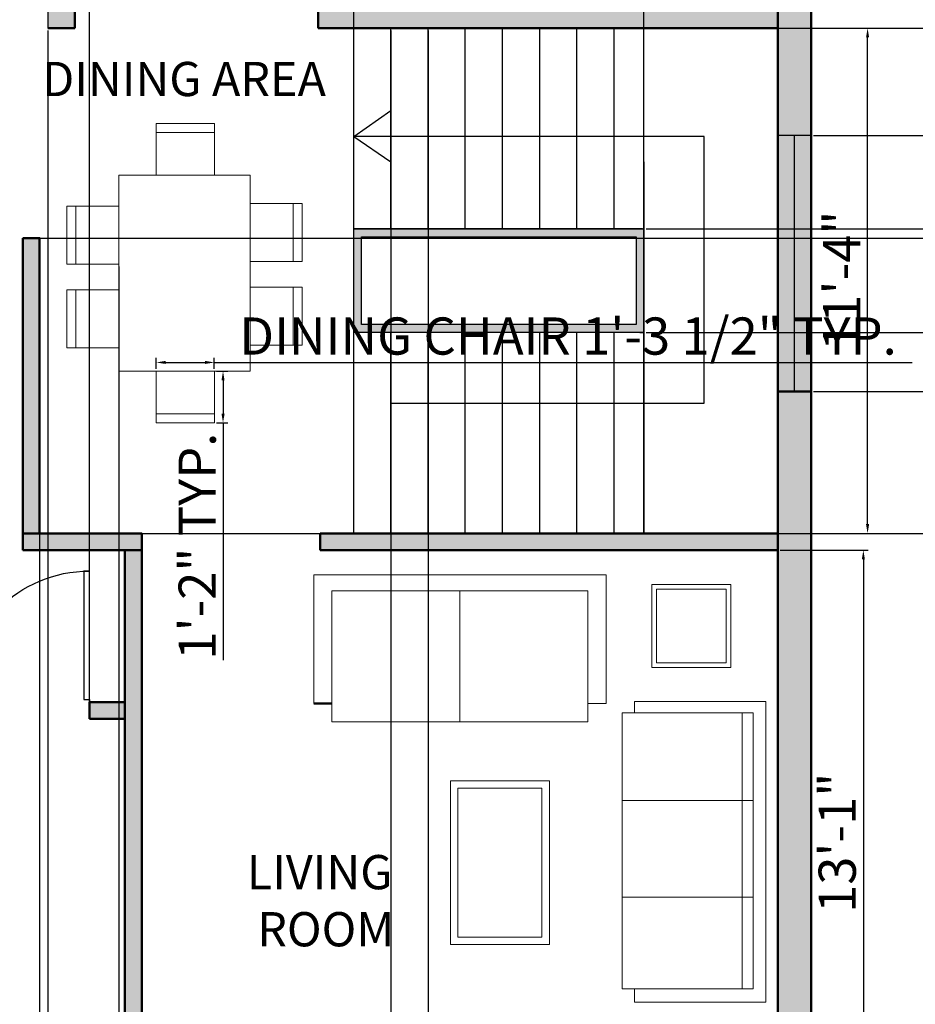
# Model space of a CAD drawing. Units: inches. Extents: x 1344 to 2521, y 3236 to 4924.
# Tile 10 of 14: x 1561 to 1801, y 4260 to 4525. Entities that reach past the tile are written whole.
import ezdxf

# ---------------------------------------------------------------- set-up
doc = ezdxf.new("R2010")
doc.units = ezdxf.units.IN
for name, color, linetype, lineweight in [('A-ANNO-DIMS', 2, 'Continuous', 18), ('A-AREA-IDEN', 3, 'Continuous', 18), ('A-DOOR', 50, 'Continuous', 25), ('A-FLOR-STRS', 7, 'Continuous', 25), ('A-FURN', 130, 'Continuous', 18), ('A-GLAZ', 150, 'Continuous', 25), ('A-WALL', 31, 'Continuous', 50), ('A-WALL-PATT', 8, 'Continuous', 13)]:
    doc.layers.add(name, color=color, linetype=linetype, lineweight=lineweight)
doc.styles.get("Standard").update_dxf_attribs({"font": 'arial.ttf'})
doc.dimstyles.new('ISO-25', dxfattribs={"dimtxt": 10, "dimasz": 2.5, "dimexe": 1.25, "dimexo": 0.625, "dimtad": 1, "dimdec": 0, "dimlunit": 4, "dimtxsty": 'Standard', "dimcen": 2.5, "dimadec": 0, "dimazin": 0, "dimtfac": 1, "dimtdec": 0, "dimtmove": 0, "dimatfit": 3, "dimfxl": 1, "dimarcsym": 0})

# ---------------------------------------------------------------- blocks, each defined once
blk = doc.blocks.new('*U2')
for p, q in [((0, 0), (0, -6)), ((40, 0), (40, -6))]:
    blk.add_line(p, q)
blk.add_lwpolyline([(0, 0), (0, 40), (1.75, 40), (1.75, 0)], close=True)
blk.add_arc((0, 0), 40, 0, 90)
blk = doc.blocks.new('*D28')
at = {"layer": 'A-ANNO-DIMS', "color": 0, "lineweight": -2, "transparency": 16777216}
for p, q in [((1765.14, 4382.64), (1788.78, 4382.64)), ((1787.53, 4380.14), (1787.53, 4227.72)), ((1765.14, 4225.22), (1788.78, 4225.22))]:
    blk.add_line(p, q, dxfattribs=at)
at = {"layer": 'A-ANNO-DIMS', "color": 0, "lineweight": 100, "transparency": 16777216}
for points in [[(1787.11, 4380.14), (1787.95, 4380.14), (1787.53, 4382.64)], [(1787.11, 4227.72), (1787.95, 4227.72), (1787.53, 4225.22)]]:
    blk.add_solid(points, dxfattribs=at)
at = {"layer": 'Defpoints', "color": 0, "lineweight": 100, "transparency": 16777216}
for p in [(1764.52, 4382.64), (1764.52, 4225.22), (1787.53, 4225.22)]:
    blk.add_point(p, dxfattribs=at)
at = {"layer": 'A-ANNO-DIMS', "color": 0, "transparency": 16777216, "insert": (1781.8, 4303.93), "char_height": 10, "attachment_point": 5, "rotation": 90}
blk.add_mtext('13\'-1"', dxfattribs=at)
blk = doc.blocks.new('*D29')
at = {"layer": 'A-ANNO-DIMS', "color": 0, "lineweight": -2, "transparency": 16777216}
for p, q in [((1765.14, 4523.04), (1789.92, 4523.04)), ((1788.67, 4389.64), (1788.67, 4520.54)), ((1765.14, 4387.14), (1789.92, 4387.14))]:
    blk.add_line(p, q, dxfattribs=at)
at = {"layer": 'A-ANNO-DIMS', "color": 0, "lineweight": 100, "transparency": 16777216}
for points in [[(1788.25, 4520.54), (1789.08, 4520.54), (1788.67, 4523.04)], [(1788.25, 4389.64), (1789.08, 4389.64), (1788.67, 4387.14)]]:
    blk.add_solid(points, dxfattribs=at)
at = {"layer": 'Defpoints', "color": 0, "lineweight": 100, "transparency": 16777216}
for p in [(1764.52, 4523.04), (1788.67, 4523.04), (1764.52, 4387.14)]:
    blk.add_point(p, dxfattribs=at)
at = {"layer": 'A-ANNO-DIMS', "color": 0, "transparency": 16777216, "insert": (1783.02, 4455.09), "char_height": 10, "attachment_point": 5, "rotation": 90}
blk.add_mtext('11\'-4"', dxfattribs=at)
blk = doc.blocks.new('DINING-CHAIR')
blk.add_line((0, 11.49), (15.6, 11.49))
blk.add_lwpolyline([(0, 0), (15.6, 0), (15.6, 13.94), (0, 13.94)], close=True)
blk = doc.blocks.new('*D67')
at = {"layer": 'A-ANNO-DIMS', "color": 0, "lineweight": -2, "transparency": 16777216}
for p, q in [((1597.45, 4431.41), (1597.45, 4434.37)), ((1599.95, 4433.12), (1610.54, 4433.12)), ((1613.04, 4431.41), (1613.04, 4434.37)), ((1613.04, 4433.12), (1800.68, 4433.12))]:
    blk.add_line(p, q, dxfattribs=at)
at = {"layer": 'A-ANNO-DIMS', "color": 0, "lineweight": 100, "transparency": 16777216}
for points in [[(1599.95, 4433.54), (1599.95, 4432.71), (1597.45, 4433.12)], [(1610.54, 4433.54), (1610.54, 4432.71), (1613.04, 4433.12)]]:
    blk.add_solid(points, dxfattribs=at)
at = {"layer": 'Defpoints', "color": 0, "lineweight": 100, "transparency": 16777216}
for p in [(1613.04, 4433.12), (1597.45, 4430.78), (1613.04, 4430.78)]:
    blk.add_point(p, dxfattribs=at)
at = {"layer": 'A-ANNO-DIMS', "color": 0, "transparency": 16777216, "insert": (1708.11, 4438.92), "char_height": 10, "attachment_point": 5}
blk.add_mtext('DINING CHAIR 1\'-3 1/2" TYP.', dxfattribs=at)
blk = doc.blocks.new('*D68')
at = {"layer": 'A-ANNO-DIMS', "color": 0, "lineweight": -2, "transparency": 16777216}
for p, q in [((1613.67, 4430.78), (1616.63, 4430.78)), ((1615.38, 4428.28), (1615.38, 4419.34)), ((1613.67, 4416.84), (1616.63, 4416.84)), ((1615.38, 4416.84), (1615.38, 4353.08))]:
    blk.add_line(p, q, dxfattribs=at)
at = {"layer": 'A-ANNO-DIMS', "color": 0, "lineweight": 100, "transparency": 16777216}
for points in [[(1614.97, 4428.28), (1615.8, 4428.28), (1615.38, 4430.78)], [(1614.97, 4419.34), (1615.8, 4419.34), (1615.38, 4416.84)]]:
    blk.add_solid(points, dxfattribs=at)
at = {"layer": 'Defpoints', "color": 0, "lineweight": 100, "transparency": 16777216}
for p in [(1613.04, 4430.78), (1613.04, 4416.84), (1615.38, 4416.84)]:
    blk.add_point(p, dxfattribs=at)
at = {"layer": 'A-ANNO-DIMS', "color": 0, "transparency": 16777216, "insert": (1609.73, 4383.71), "char_height": 10, "attachment_point": 5, "rotation": 90}
blk.add_mtext('1\'-2" TYP.', dxfattribs=at)
blk = doc.blocks.new('*D87')
at = {"layer": 'A-ANNO-DIMS', "color": 0, "lineweight": -2, "transparency": 16777216}
for p, q in [((1774.14, 4560.16), (1820.02, 4560.16)), ((1818.77, 4557.66), (1818.77, 4496.69)), ((1774.14, 4494.19), (1820.02, 4494.19))]:
    blk.add_line(p, q, dxfattribs=at)
at = {"layer": 'A-ANNO-DIMS', "color": 0, "lineweight": 100, "transparency": 16777216}
for points in [[(1818.35, 4557.66), (1819.18, 4557.66), (1818.77, 4560.16)], [(1818.35, 4496.69), (1819.18, 4496.69), (1818.77, 4494.19)]]:
    blk.add_solid(points, dxfattribs=at)
at = {"layer": 'Defpoints', "color": 0, "lineweight": 100, "transparency": 16777216}
for p in [(1773.52, 4560.16), (1773.52, 4494.19), (1818.77, 4494.19)]:
    blk.add_point(p, dxfattribs=at)
at = {"layer": 'A-ANNO-DIMS', "color": 0, "transparency": 16777216, "insert": (1813.04, 4527.17), "char_height": 10, "attachment_point": 5, "rotation": 90}
blk.add_mtext('5\'-6"', dxfattribs=at)
blk = doc.blocks.new('*D88')
at = {"layer": 'A-ANNO-DIMS', "color": 0, "lineweight": -2, "transparency": 16777216}
for p, q in [((1774.14, 4494.19), (1820.02, 4494.19)), ((1818.77, 4491.69), (1818.77, 4427.77)), ((1774.14, 4425.27), (1820.02, 4425.27))]:
    blk.add_line(p, q, dxfattribs=at)
at = {"layer": 'A-ANNO-DIMS', "color": 0, "lineweight": 100, "transparency": 16777216}
for points in [[(1818.35, 4491.69), (1819.18, 4491.69), (1818.77, 4494.19)], [(1818.35, 4427.77), (1819.18, 4427.77), (1818.77, 4425.27)]]:
    blk.add_solid(points, dxfattribs=at)
at = {"layer": 'Defpoints', "color": 0, "lineweight": 100, "transparency": 16777216}
for p in [(1773.52, 4494.19), (1773.52, 4425.27), (1818.77, 4425.27)]:
    blk.add_point(p, dxfattribs=at)
at = {"layer": 'A-ANNO-DIMS', "color": 0, "transparency": 16777216, "insert": (1813.04, 4459.73), "char_height": 10, "attachment_point": 5, "rotation": 90}
blk.add_mtext('5\'-9"', dxfattribs=at)
blk = doc.blocks.new('*D89')
at = {"layer": 'A-ANNO-DIMS', "color": 0, "lineweight": -2, "transparency": 16777216}
for p, q in [((1774.14, 4425.27), (1820.02, 4425.27)), ((1818.77, 4422.77), (1818.77, 4155.71)), ((1774.14, 4153.21), (1820.02, 4153.21))]:
    blk.add_line(p, q, dxfattribs=at)
at = {"layer": 'A-ANNO-DIMS', "color": 0, "lineweight": 100, "transparency": 16777216}
for points in [[(1818.35, 4422.77), (1819.18, 4422.77), (1818.77, 4425.27)], [(1818.35, 4155.71), (1819.18, 4155.71), (1818.77, 4153.21)]]:
    blk.add_solid(points, dxfattribs=at)
at = {"layer": 'Defpoints', "color": 0, "lineweight": 100, "transparency": 16777216}
for p in [(1773.52, 4425.27), (1773.52, 4153.21), (1818.77, 4153.21)]:
    blk.add_point(p, dxfattribs=at)
at = {"layer": 'A-ANNO-DIMS', "color": 0, "transparency": 16777216, "insert": (1813.04, 4289.24), "char_height": 10, "attachment_point": 5, "rotation": 90}
blk.add_mtext('22\'-8"', dxfattribs=at)
blk = doc.blocks.new('*D93')
at = {"layer": 'A-ANNO-DIMS', "color": 0, "lineweight": -2, "transparency": 16777216}
for p, q in [((1526.04, 4667.09), (1526.04, 4106.71)), ((1557.42, 4667.09), (1557.42, 4106.71)), ((1528.54, 4107.96), (1554.92, 4107.96)), ((1557.42, 4107.96), (1611.23, 4107.96))]:
    blk.add_line(p, q, dxfattribs=at)
at = {"layer": 'A-ANNO-DIMS', "color": 0, "lineweight": 100, "transparency": 16777216}
for points in [[(1528.54, 4108.38), (1528.54, 4107.54), (1526.04, 4107.96)], [(1554.92, 4108.38), (1554.92, 4107.54), (1557.42, 4107.96)]]:
    blk.add_solid(points, dxfattribs=at)
at = {"layer": 'Defpoints', "color": 0, "lineweight": 100, "transparency": 16777216}
for p in [(1526.04, 4667.71), (1557.42, 4667.71), (1557.42, 4107.96)]:
    blk.add_point(p, dxfattribs=at)
at = {"layer": 'A-ANNO-DIMS', "color": 0, "transparency": 16777216, "insert": (1585.57, 4113.76), "char_height": 10, "attachment_point": 5}
blk.add_mtext('2\'-7 1/2"', dxfattribs=at)
blk = doc.blocks.new('*D95')
at = {"layer": 'A-ANNO-DIMS', "color": 0, "lineweight": -2, "transparency": 16777216}
for p, q in [((1528.27, 4522.42), (1528.27, 4106.71)), ((1568.27, 4522.42), (1568.27, 4106.71)), ((1530.77, 4107.96), (1565.77, 4107.96))]:
    blk.add_line(p, q, dxfattribs=at)
at = {"layer": 'A-ANNO-DIMS', "color": 0, "lineweight": 100, "transparency": 16777216}
for points in [[(1530.77, 4108.38), (1530.77, 4107.54), (1528.27, 4107.96)], [(1565.77, 4108.38), (1565.77, 4107.54), (1568.27, 4107.96)]]:
    blk.add_solid(points, dxfattribs=at)
at = {"layer": 'Defpoints', "color": 0, "lineweight": 100, "transparency": 16777216}
for p in [(1528.27, 4523.04), (1568.27, 4523.04), (1568.27, 4107.96)]:
    blk.add_point(p, dxfattribs=at)
at = {"layer": 'A-ANNO-DIMS', "color": 0, "transparency": 16777216, "insert": (1548.27, 4113.7), "char_height": 10, "attachment_point": 5}
blk.add_mtext('3\'-4"', dxfattribs=at)
blk = doc.blocks.new('*D97')
at = {"layer": 'A-ANNO-DIMS', "color": 0, "lineweight": -2, "transparency": 16777216}
for p, q in [((1566.07, 4465.94), (1566.07, 4106.71)), ((1587.33, 4458.96), (1587.33, 4106.71)), ((1568.57, 4107.96), (1584.83, 4107.96)), ((1587.33, 4107.96), (1640.02, 4107.96))]:
    blk.add_line(p, q, dxfattribs=at)
at = {"layer": 'A-ANNO-DIMS', "color": 0, "lineweight": 100, "transparency": 16777216}
for points in [[(1568.57, 4108.38), (1568.57, 4107.54), (1566.07, 4107.96)], [(1584.83, 4108.38), (1584.83, 4107.54), (1587.33, 4107.96)]]:
    blk.add_solid(points, dxfattribs=at)
at = {"layer": 'Defpoints', "color": 0, "lineweight": 100, "transparency": 16777216}
for p in [(1566.07, 4466.57), (1587.33, 4459.59), (1587.33, 4107.96)]:
    blk.add_point(p, dxfattribs=at)
at = {"layer": 'A-ANNO-DIMS', "color": 0, "transparency": 16777216, "insert": (1614.92, 4113.76), "char_height": 10, "attachment_point": 5}
blk.add_mtext('1\'-9 1/2"', dxfattribs=at)
blk = doc.blocks.new('*D98')
at = {"layer": 'A-ANNO-DIMS', "color": 0, "lineweight": -2, "transparency": 16777216}
for p, q in [((1562.2, 4466.57), (1820.02, 4466.57)), ((1818.77, 4464.07), (1818.77, 4389.64)), ((1562.2, 4387.14), (1820.02, 4387.14))]:
    blk.add_line(p, q, dxfattribs=at)
at = {"layer": 'A-ANNO-DIMS', "color": 0, "lineweight": 100, "transparency": 16777216}
for points in [[(1818.35, 4464.07), (1819.18, 4464.07), (1818.77, 4466.57)], [(1818.35, 4389.64), (1819.18, 4389.64), (1818.77, 4387.14)]]:
    blk.add_solid(points, dxfattribs=at)
at = {"layer": 'Defpoints', "color": 0, "lineweight": 100, "transparency": 16777216}
for p in [(1561.57, 4466.57), (1561.57, 4387.14), (1818.77, 4387.14)]:
    blk.add_point(p, dxfattribs=at)
at = {"layer": 'A-ANNO-DIMS', "color": 0, "transparency": 16777216, "insert": (1812.97, 4426.85), "char_height": 10, "attachment_point": 5, "rotation": 90}
blk.add_mtext('6\'-7 1/2"', dxfattribs=at)
blk = doc.blocks.new('*D99')
at = {"layer": 'A-ANNO-DIMS', "color": 0, "lineweight": -2, "transparency": 16777216}
for p, q in [((1544.94, 4337.92), (1544.94, 4850.71)), ((1547.44, 4849.46), (1577, 4849.46)), ((1579.5, 4337.92), (1579.5, 4850.71)), ((1579.5, 4849.46), (1641.07, 4849.46))]:
    blk.add_line(p, q, dxfattribs=at)
at = {"layer": 'A-ANNO-DIMS', "color": 0, "lineweight": 100, "transparency": 16777216}
for points in [[(1547.44, 4849.88), (1547.44, 4849.04), (1544.94, 4849.46)], [(1577, 4849.88), (1577, 4849.04), (1579.5, 4849.46)]]:
    blk.add_solid(points, dxfattribs=at)
at = {"layer": 'Defpoints', "color": 0, "lineweight": 100, "transparency": 16777216}
for p in [(1579.5, 4849.46), (1544.94, 4337.29), (1579.5, 4337.29)]:
    blk.add_point(p, dxfattribs=at)
at = {"layer": 'A-ANNO-DIMS', "color": 0, "transparency": 16777216, "insert": (1611.53, 4855.26), "char_height": 10, "attachment_point": 5}
blk.add_mtext('2\'-10 1/2"', dxfattribs=at)
blk = doc.blocks.new('*D100')
at = {"layer": 'A-ANNO-DIMS', "color": 0, "lineweight": -2, "transparency": 16777216}
for p, q in [((1660.52, 4522.42), (1660.52, 4106.71)), ((1670.52, 4522.42), (1670.52, 4106.71)), ((1663.02, 4107.96), (1668.02, 4107.96)), ((1670.52, 4107.96), (1708.62, 4107.96))]:
    blk.add_line(p, q, dxfattribs=at)
at = {"layer": 'A-ANNO-DIMS', "color": 0, "lineweight": 100, "transparency": 16777216}
for points in [[(1663.02, 4108.38), (1663.02, 4107.54), (1660.52, 4107.96)], [(1668.02, 4108.38), (1668.02, 4107.54), (1670.52, 4107.96)]]:
    blk.add_solid(points, dxfattribs=at)
at = {"layer": 'Defpoints', "color": 0, "lineweight": 100, "transparency": 16777216}
for p in [(1660.52, 4523.04), (1670.52, 4523.04), (1670.52, 4107.96)]:
    blk.add_point(p, dxfattribs=at)
at = {"layer": 'A-ANNO-DIMS', "color": 0, "transparency": 16777216, "insert": (1690.82, 4113.69), "char_height": 10, "attachment_point": 5}
blk.add_mtext('0\'-10"', dxfattribs=at)
blk = doc.blocks.new('*D101')
at = {"layer": 'A-ANNO-DIMS', "color": 0, "lineweight": -2, "transparency": 16777216}
for p, q in [((1650.52, 4387.77), (1650.52, 4850.71)), ((1653.02, 4849.46), (1726.02, 4849.46)), ((1728.52, 4387.77), (1728.52, 4850.71))]:
    blk.add_line(p, q, dxfattribs=at)
at = {"layer": 'A-ANNO-DIMS', "color": 0, "lineweight": 100, "transparency": 16777216}
for points in [[(1653.02, 4849.88), (1653.02, 4849.04), (1650.52, 4849.46)], [(1726.02, 4849.88), (1726.02, 4849.04), (1728.52, 4849.46)]]:
    blk.add_solid(points, dxfattribs=at)
at = {"layer": 'Defpoints', "color": 0, "lineweight": 100, "transparency": 16777216}
for p in [(1728.52, 4849.46), (1650.52, 4387.14), (1728.52, 4387.14)]:
    blk.add_point(p, dxfattribs=at)
at = {"layer": 'A-ANNO-DIMS', "color": 0, "transparency": 16777216, "insert": (1689.52, 4855.19), "char_height": 10, "attachment_point": 5}
blk.add_mtext('6\'-6"', dxfattribs=at)
blk = doc.blocks.new('*D102')
at = {"layer": 'A-ANNO-DIMS', "color": 0, "lineweight": -2, "transparency": 16777216}
for p, q in [((1728.52, 4387.77), (1728.52, 4850.71)), ((1731.02, 4849.46), (1762.02, 4849.46)), ((1764.52, 4387.77), (1764.52, 4850.71))]:
    blk.add_line(p, q, dxfattribs=at)
at = {"layer": 'A-ANNO-DIMS', "color": 0, "lineweight": 100, "transparency": 16777216}
for points in [[(1731.02, 4849.88), (1731.02, 4849.04), (1728.52, 4849.46)], [(1762.02, 4849.88), (1762.02, 4849.04), (1764.52, 4849.46)]]:
    blk.add_solid(points, dxfattribs=at)
at = {"layer": 'Defpoints', "color": 0, "lineweight": 100, "transparency": 16777216}
for p in [(1764.52, 4849.46), (1728.52, 4387.14), (1764.52, 4387.14)]:
    blk.add_point(p, dxfattribs=at)
at = {"layer": 'A-ANNO-DIMS', "color": 0, "transparency": 16777216, "insert": (1746.52, 4855.2), "char_height": 10, "attachment_point": 5}
blk.add_mtext('3\'-0"', dxfattribs=at)
blk = doc.blocks.new('*D103')
at = {"layer": 'A-ANNO-DIMS', "color": 0, "lineweight": -2, "transparency": 16777216}
for p, q in [((1729.14, 4441.19), (1820.02, 4441.19)), ((1818.77, 4389.64), (1818.77, 4438.69)), ((1729.14, 4387.14), (1820.02, 4387.14))]:
    blk.add_line(p, q, dxfattribs=at)
at = {"layer": 'A-ANNO-DIMS', "color": 0, "lineweight": 100, "transparency": 16777216}
for points in [[(1818.35, 4438.69), (1819.18, 4438.69), (1818.77, 4441.19)], [(1818.35, 4389.64), (1819.18, 4389.64), (1818.77, 4387.14)]]:
    blk.add_solid(points, dxfattribs=at)
at = {"layer": 'Defpoints', "color": 0, "lineweight": 100, "transparency": 16777216}
for p in [(1728.52, 4441.19), (1818.77, 4441.19), (1728.52, 4387.14)]:
    blk.add_point(p, dxfattribs=at)
at = {"layer": 'A-ANNO-DIMS', "color": 0, "transparency": 16777216, "insert": (1813.04, 4414.17), "char_height": 10, "attachment_point": 5, "rotation": 90}
blk.add_mtext('4\'-6"', dxfattribs=at)
blk = doc.blocks.new('*D104')
at = {"layer": 'A-ANNO-DIMS', "color": 0, "lineweight": -2, "transparency": 16777216}
for p, q in [((1818.77, 4469.04), (1818.77, 4499.54)), ((1729.14, 4469.04), (1820.02, 4469.04)), ((1818.77, 4443.69), (1818.77, 4466.54)), ((1729.14, 4441.19), (1820.02, 4441.19))]:
    blk.add_line(p, q, dxfattribs=at)
at = {"layer": 'A-ANNO-DIMS', "color": 0, "lineweight": 100, "transparency": 16777216}
for points in [[(1818.35, 4466.54), (1819.18, 4466.54), (1818.77, 4469.04)], [(1818.35, 4443.69), (1819.18, 4443.69), (1818.77, 4441.19)]]:
    blk.add_solid(points, dxfattribs=at)
at = {"layer": 'Defpoints', "color": 0, "lineweight": 100, "transparency": 16777216}
for p in [(1728.52, 4469.04), (1818.77, 4469.04), (1728.52, 4441.19)]:
    blk.add_point(p, dxfattribs=at)
at = {"layer": 'A-ANNO-DIMS', "color": 0, "transparency": 16777216, "insert": (1813.12, 4485.54), "char_height": 10, "attachment_point": 5, "rotation": 90}
blk.add_mtext('2\'-4"', dxfattribs=at)
blk = doc.blocks.new('*D105')
at = {"layer": 'A-ANNO-DIMS', "color": 0, "lineweight": -2, "transparency": 16777216}
for p, q in [((1729.14, 4523.04), (1820.02, 4523.04)), ((1818.77, 4471.54), (1818.77, 4520.54)), ((1729.14, 4469.04), (1820.02, 4469.04))]:
    blk.add_line(p, q, dxfattribs=at)
at = {"layer": 'A-ANNO-DIMS', "color": 0, "lineweight": 100, "transparency": 16777216}
for points in [[(1818.35, 4520.54), (1819.18, 4520.54), (1818.77, 4523.04)], [(1818.35, 4471.54), (1819.18, 4471.54), (1818.77, 4469.04)]]:
    blk.add_solid(points, dxfattribs=at)
at = {"layer": 'Defpoints', "color": 0, "lineweight": 100, "transparency": 16777216}
for p in [(1728.52, 4523.04), (1818.77, 4523.04), (1728.52, 4469.04)]:
    blk.add_point(p, dxfattribs=at)
at = {"layer": 'A-ANNO-DIMS', "color": 0, "transparency": 16777216, "insert": (1813.04, 4496.04), "char_height": 10, "attachment_point": 5, "rotation": 90}
blk.add_mtext('4\'-6"', dxfattribs=at)

msp = doc.modelspace()

# ---------------------------------------------------------------- hatches: boundary and pattern name
at = {"layer": 'A-WALL-PATT'}
h = msp.add_hatch(color=256, dxfattribs=at)
h.dxf.hatch_style = 1
h.paths.add_polyline_path([(1595.66, 4753.21), (1558.43, 4753.21), (1558.43, 4744.21), (1571.02, 4744.21), (1595.66, 4744.21)])
h.paths.add_polyline_path([(1681.23, 4753.21), (1626.69, 4753.21), (1626.69, 4744.21), (1681.23, 4744.21)])
h.paths.add_polyline_path([(1773.52, 4753.21), (1712.26, 4753.21), (1712.26, 4744.21), (1764.52, 4744.21), (1764.52, 4629.08), (1773.52, 4629.08)])
h.paths.add_polyline_path([(1527.4, 4753.21), (1476.83, 4753.21), (1476.83, 4744.21), (1518.52, 4744.21), (1527.4, 4744.21)])
h.paths.add_polyline_path([(1445.8, 4753.21), (1413.52, 4753.21), (1413.52, 4639.46), (1422.52, 4639.46), (1422.52, 4744.21), (1445.8, 4744.21)])
h.paths.add_polyline_path([(1523.02, 4744.21), (1518.52, 4744.21), (1518.52, 4672.21), (1515.66, 4672.21), (1515.66, 4667.71), (1523.02, 4667.71), (1526.04, 4667.71), (1526.04, 4672.21), (1523.02, 4672.21)])
h.paths.add_polyline_path([(1575.52, 4744.21), (1571.02, 4744.21), (1571.02, 4672.21), (1557.42, 4672.21), (1557.42, 4667.71), (1571.02, 4667.71), (1571.02, 4626.56), (1590.95, 4626.56), (1590.95, 4631.06), (1575.52, 4631.06), (1575.52, 4667.71)])
h.paths.add_polyline_path([(1484.28, 4672.21), (1422.52, 4672.21), (1422.52, 4667.71), (1484.28, 4667.71)])
h.paths.add_polyline_path([(1645.44, 4673.7), (1640.94, 4673.7), (1640.94, 4631.06), (1626.4, 4631.06), (1626.4, 4626.56), (1645.44, 4626.56)])
h.paths.add_polyline_path([(1645.44, 4744.21), (1640.94, 4744.21), (1640.94, 4713.7), (1645.44, 4713.7)])
h.paths.add_polyline_path([(1764.52, 4671), (1645.44, 4671), (1645.44, 4666.5), (1764.52, 4666.5)])
h.paths.add_polyline_path([(1764.52, 4527.54), (1640.94, 4527.54), (1640.94, 4523.04), (1764.52, 4523.04)])
h.paths.add_polyline_path([(1645.44, 4555.81), (1645.44, 4559.03), (1640.94, 4559.03), (1640.94, 4527.54), (1645.44, 4527.54)])
h = msp.add_hatch(color=256, dxfattribs=at)
h.dxf.hatch_style = 1
h.paths.add_polyline_path([(1773.52, 4425.27), (1764.52, 4425.27), (1764.52, 4225.22), (1743.16, 4225.22), (1743.16, 4216.22), (1764.52, 4216.22), (1764.52, 4162.21), (1764.52, 4155.88), (1653.6, 4155.88), (1653.6, 4177.58), (1764.52, 4177.58), (1764.52, 4180.4), (1649.25, 4180.4), (1649.25, 4153.21), (1773.52, 4153.21)], flags=17)
h.paths.add_polyline_path([(1598.02, 4180.38), (1593.52, 4180.38), (1589.02, 4180.38), (1589.02, 4162.21), (1565.92, 4162.21), (1565.92, 4153.21), (1598.02, 4153.21)], flags=17)
h.paths.add_polyline_path([(1689.47, 4225.22), (1666.04, 4225.22), (1666.04, 4220.75), (1666.04, 4216.22), (1689.47, 4216.22)], flags=16)
h.paths.add_polyline_path([(1442.43, 4162.21), (1422.52, 4162.21), (1422.52, 4744.21), (1764.52, 4744.21), (1764.52, 4225.22), (1743.16, 4225.22), (1743.16, 4216.22), (1764.52, 4216.22), (1764.52, 4162.21), (1764.52, 4155.88), (1653.6, 4155.88), (1653.6, 4177.58), (1764.52, 4177.58), (1764.52, 4180.4), (1649.25, 4180.4), (1649.25, 4153.21), (1773.52, 4153.21), (1773.52, 4425.27), (1773.52, 4753.21), (1413.52, 4753.21), (1413.52, 4153.21), (1442.43, 4153.21)])
h.paths.add_polyline_path([(1648.69, 4179.48), (1724.08, 4179.48), (1724.08, 4213.98), (1648.69, 4213.98)], flags=25)
h.paths.add_polyline_path([(1609.51, 4245.39), (1659.17, 4245.39), (1659.17, 4264.37), (1609.51, 4264.37)], flags=25)
h.paths.add_polyline_path([(1618.52, 4270.74), (1667.67, 4270.74), (1667.67, 4305.24), (1618.52, 4305.24)], flags=25)
h.paths.add_polyline_path([(1563.46, 4499.55), (1651.73, 4499.55), (1651.73, 4518.53), (1563.46, 4518.53)], flags=25)
h.paths.add_polyline_path([(1439.72, 4433.21), (1521.54, 4433.21), (1521.54, 4467.71), (1439.72, 4467.71)], flags=25)
h.paths.add_polyline_path([(1651.43, 4581.89), (1735.04, 4581.89), (1735.04, 4616.38), (1651.43, 4616.38)], flags=25)
h.paths.add_polyline_path([(1495.42, 4585.56), (1566.53, 4585.56), (1566.53, 4620.06), (1495.42, 4620.06)], flags=25)
h.paths.add_polyline_path([(1677.05, 4699.47), (1729.56, 4699.47), (1729.56, 4718.45), (1677.05, 4718.45)], flags=25)
h.paths.add_polyline_path([(1581.37, 4669.39), (1626.01, 4669.39), (1626.01, 4703.88), (1581.37, 4703.88)], flags=25)
h.paths.add_polyline_path([(1523.21, 4717.23), (1572.85, 4717.23), (1572.85, 4736.21), (1523.21, 4736.21)], flags=25)
h.paths.add_polyline_path([(1432.59, 4685.86), (1482.24, 4685.86), (1482.24, 4704.84), (1432.59, 4704.84)], flags=25)
h = msp.add_hatch(color=256, dxfattribs=at)
h.dxf.hatch_style = 1
h.paths.add_polyline_path([(1528.27, 4527.54), (1422.52, 4527.54), (1422.52, 4523.04), (1499.65, 4523.04), (1528.27, 4523.04)])
h.paths.add_polyline_path([(1575.52, 4626.56), (1571.02, 4626.56), (1571.02, 4527.54), (1568.27, 4527.54), (1568.27, 4523.04), (1575.52, 4523.04)])
h.paths.add_polyline_path([(1413.52, 4445.6), (1422.52, 4445.6), (1422.52, 4570.54), (1413.52, 4570.54)])
h = msp.add_hatch(color=256, dxfattribs=at)
h.dxf.hatch_style = 1
h.paths.add_polyline_path([(1764.52, 4382.64), (1764.52, 4387.14), (1641.52, 4387.14), (1641.52, 4382.64)])
h.paths.add_polyline_path([(1650.52, 4441.19), (1728.52, 4441.19), (1728.52, 4469.04), (1650.52, 4469.04)])
h.paths.add_polyline_path([(1726.41, 4466.94), (1726.41, 4443.29), (1652.62, 4443.29), (1652.62, 4466.94)], flags=16)
h = msp.add_hatch(color=256, dxfattribs=at)
h.dxf.hatch_style = 1
h.paths.add_polyline_path([(1773.52, 4215.79), (1764.52, 4215.79), (1764.52, 4153.21), (1773.52, 4153.21)])
h.paths.add_polyline_path([(1773.52, 4425.27), (1764.52, 4425.27), (1764.52, 4216.22), (1773.52, 4216.22)])
h.paths.add_polyline_path([(1764.52, 4225.22), (1743.16, 4225.22), (1743.16, 4216.22), (1764.52, 4216.22)])
h.paths.add_polyline_path([(1764.52, 4180.4), (1649.25, 4180.4), (1649.25, 4153.21), (1764.52, 4153.21), (1764.52, 4155.88), (1653.6, 4155.88), (1653.6, 4177.58), (1764.52, 4177.58)])
h.paths.add_polyline_path([(1605.63, 4225.22), (1589.02, 4225.22), (1589.02, 4216.22), (1605.63, 4216.22)])
h.paths.add_polyline_path([(1593.52, 4382.64), (1589.02, 4382.64), (1589.02, 4225.22), (1593.52, 4225.22)])
h.paths.add_polyline_path([(1544.94, 4341.79), (1422.52, 4341.79), (1422.52, 4337.29), (1544.94, 4337.29)])
h.paths.add_polyline_path([(1593.52, 4387.14), (1561.57, 4387.14), (1561.57, 4382.64), (1593.52, 4382.64)])
h.paths.add_polyline_path([(1566.07, 4466.57), (1561.57, 4466.57), (1561.57, 4387.14), (1566.07, 4387.14)])
h = msp.add_hatch(color=256, dxfattribs=at)
h.dxf.hatch_style = 1
h.paths.add_polyline_path([(1589.02, 4337.29), (1589.02, 4341.79), (1579.5, 4341.79), (1579.5, 4337.29)])

# ---------------------------------------------------------------- linework, layer by layer
at = {"layer": 'A-FLOR-STRS'}
for p, q in [((1650.52, 4387.14), (1650.52, 4523.04)), ((1660.52, 4475.04), (1660.52, 4523.04)), ((1670.52, 4475.04), (1670.52, 4523.04)), ((1680.52, 4475.04), (1680.52, 4523.04)), ((1690.52, 4475.04), (1690.52, 4523.04)), ((1700.52, 4475.04), (1700.52, 4523.04)), ((1710.52, 4475.04), (1710.52, 4523.04)), ((1720.52, 4475.04), (1720.52, 4523.04)), ((1728.52, 4387.14), (1728.52, 4523.04)), ((1650.52, 4493.89), (1660.52, 4500.89)), ((1744.72, 4493.89), (1650.52, 4493.89)), ((1650.52, 4493.89), (1660.52, 4487.1)), ((1744.72, 4422.14), (1744.72, 4493.89)), ((1660.52, 4469.04), (1660.52, 4489.35)), ((1728.52, 4487.04), (1728.52, 4423.14)), ((1670.52, 4469.04), (1670.52, 4475.04)), ((1680.52, 4469.04), (1680.52, 4475.04)), ((1690.52, 4469.04), (1690.52, 4475.04)), ((1700.52, 4469.04), (1700.52, 4475.04)), ((1710.52, 4469.04), (1710.52, 4475.04)), ((1720.52, 4469.04), (1720.52, 4476.51)), ((1728.17, 4469.04), (1650.52, 4469.04)), ((1651.57, 4441.19), (1650.52, 4441.19)), ((1727.46, 4441.19), (1651.57, 4441.19)), ((1660.52, 4435.14), (1660.52, 4441.19)), ((1670.52, 4435.14), (1670.52, 4441.19)), ((1680.52, 4435.14), (1680.52, 4441.19)), ((1690.52, 4435.14), (1690.52, 4441.19)), ((1700.52, 4435.14), (1700.52, 4441.19)), ((1710.52, 4435.14), (1710.52, 4441.19)), ((1720.52, 4435.14), (1720.52, 4441.19)), ((1727.46, 4441.19), (1728.52, 4441.19)), ((1660.52, 4387.14), (1660.52, 4435.14)), ((1670.52, 4387.14), (1670.52, 4435.14)), ((1680.52, 4387.14), (1680.52, 4435.14)), ((1690.52, 4387.14), (1690.52, 4435.14)), ((1700.52, 4387.14), (1700.52, 4435.14)), ((1710.52, 4387.14), (1710.52, 4435.14)), ((1720.52, 4387.14), (1720.52, 4435.14)), ((1660.52, 4422.14), (1744.72, 4422.14)), ((1728.52, 4423.14), (1728.52, 4387.14))]:
    msp.add_line(p, q, dxfattribs=at)
for points in [[(1650.52, 4469.04), (1728.52, 4469.04), (1728.52, 4441.19), (1650.52, 4441.19)], [(1652.62, 4466.94), (1726.41, 4466.94), (1726.41, 4443.29), (1652.62, 4443.29)]]:
    msp.add_lwpolyline(points, close=True, dxfattribs=at)
at = {"layer": 'A-FURN'}
for p, q in [((1639.76, 4341.39), (1639.76, 4375.98)), ((1639.76, 4375.98), (1718.38, 4375.98)), ((1718.38, 4375.98), (1718.38, 4341.39)), ((1679.04, 4336.48), (1679.04, 4371.72)), ((1718.38, 4341.39), (1713.47, 4341.39)), ((1726.01, 4338.87), (1726.01, 4341.89)), ((1726.01, 4341.89), (1761.35, 4341.89)), ((1761.35, 4341.89), (1761.35, 4261.04)), ((1754.94, 4264.65), (1754.94, 4338.87)), ((1757.91, 4315.28), (1722.72, 4315.28)), ((1757.91, 4289.28), (1722.72, 4289.28)), ((1726.01, 4261.04), (1726.01, 4264.65)), ((1761.35, 4261.04), (1726.01, 4261.04))]:
    msp.add_line(p, q, dxfattribs=at)
for points in [[(1587.33, 4483.47), (1622.72, 4483.47), (1622.72, 4430.78), (1587.33, 4430.78)], [(1730.67, 4351.07), (1751.92, 4351.07), (1751.92, 4373.42), (1730.67, 4373.42)], [(1731.92, 4352.33), (1750.66, 4352.33), (1750.66, 4372.17), (1731.92, 4372.17)], [(1713.47, 4336.48), (1644.61, 4336.48), (1644.61, 4371.72), (1713.47, 4371.72)], [(1757.91, 4338.87), (1722.72, 4338.87), (1722.72, 4264.65), (1757.91, 4264.65)], [(1703.12, 4320.59), (1676.54, 4320.59), (1676.54, 4276.57), (1703.12, 4276.57)], [(1701.12, 4318.59), (1678.54, 4318.59), (1678.54, 4278.57), (1701.12, 4278.57)]]:
    msp.add_lwpolyline(points, close=True, dxfattribs=at)
at = {"layer": 'A-GLAZ'}
msp.add_line((1769.02, 4425.27), (1769.02, 4494.19), dxfattribs=at)
msp.add_lwpolyline([(1764.52, 4425.27), (1773.52, 4425.27), (1773.52, 4494.19), (1764.52, 4494.19)], close=True, dxfattribs=at)
at = {"layer": 'A-WALL'}
for p, q in [((1575.52, 4626.56), (1575.52, 4523.04)), ((1640.94, 4527.54), (1640.94, 4523.04)), ((1575.52, 4523.04), (1568.27, 4523.04)), ((1640.94, 4523.04), (1764.52, 4523.04)), ((1764.52, 4523.04), (1728.52, 4523.04)), ((1764.52, 4523.04), (1764.52, 4487.04)), ((1561.57, 4382.64), (1561.57, 4466.57)), ((1566.07, 4466.57), (1561.57, 4466.57)), ((1566.07, 4387.14), (1566.07, 4466.57)), ((1764.52, 4387.14), (1764.52, 4423.14)), ((1593.52, 4387.14), (1566.07, 4387.14)), ((1593.52, 4382.64), (1593.52, 4387.14)), ((1764.52, 4387.14), (1641.52, 4387.14)), ((1641.52, 4382.64), (1641.52, 4387.14)), ((1589.02, 4382.64), (1561.57, 4382.64)), ((1589.02, 4162.21), (1589.02, 4382.64)), ((1593.52, 4225.22), (1593.52, 4382.64)), ((1764.52, 4382.64), (1641.52, 4382.64)), ((1579.5, 4341.79), (1589.02, 4341.79)), ((1644.61, 4341.39), (1639.76, 4341.39)), ((1579.5, 4337.29), (1589.02, 4337.29))]:
    msp.add_line(p, q, dxfattribs=at)
for points in [[(1565.92, 4153.21), (1773.52, 4153.21), (1773.52, 4753.21), (1413.52, 4753.21), (1413.52, 4153.21), (1442.43, 4153.21)], [(1764.52, 4225.22), (1764.52, 4744.21), (1422.52, 4744.21), (1422.52, 4162.21), (1442.43, 4162.21)]]:
    msp.add_lwpolyline(points, dxfattribs=at)
for points in [[(1561.57, 4466.57), (1566.07, 4466.57), (1566.07, 4387.14), (1561.57, 4387.14)], [(1764.52, 4425.27), (1773.52, 4425.27), (1773.52, 4215.79), (1764.52, 4215.79)], [(1561.57, 4382.64), (1593.52, 4382.64), (1593.52, 4387.14), (1561.57, 4387.14)], [(1589.02, 4382.64), (1593.52, 4382.64), (1593.52, 4225.22), (1589.02, 4225.22)], [(1579.5, 4337.29), (1589.02, 4337.29), (1589.02, 4341.79), (1579.5, 4341.79)]]:
    msp.add_lwpolyline(points, close=True, dxfattribs=at)

# ---------------------------------------------------------------- block references
at = {"layer": 'A-DOOR', "xscale": -1}
msp.add_blockref('*U2', (1568.27, 4529.04), dxfattribs=at)
at = {"layer": 'A-DOOR', "xscale": -0.8638279890898501, "yscale": 0.8638279890898501, "zscale": 0.8638279890898501}
msp.add_blockref('*U2', (1579.5, 4342.47), dxfattribs=at)
at = {"layer": 'A-FURN'}
msp.add_blockref('DINING-CHAIR', (1597.45, 4483.47), dxfattribs=at)
at = {"layer": 'A-FURN', "extrusion": (0, 0, -1), "zscale": -1}
for p, rotation in [((-1587.33, 4475.18), 269.9999999999972), ((-1587.33, 4452.62), 270), ((-1597.45, 4430.78), 180)]:
    msp.add_blockref('DINING-CHAIR', p, dxfattribs=dict(at, rotation=rotation))
at = {"layer": 'A-FURN'}
for p, rotation in [((1622.72, 4475.9), 270), ((1622.72, 4453.33), 269.9999999999972)]:
    msp.add_blockref('DINING-CHAIR', p, dxfattribs=dict(at, rotation=rotation))

# ---------------------------------------------------------------- texts
at = {"layer": 'A-AREA-IDEN', "char_height": 9.211, "attachment_point": 1}
for s, insert in [('DINING AREA', (1566.75, 4513.95)), ('LIVING\\P ROOM', (1621.77, 4300.65))]:
    msp.add_mtext_dynamic_manual_height_columns(s, width=108.7809, gutter_width=46.06, heights=[0], dxfattribs=dict(at, insert=insert))

# ---------------------------------------------------------------- dimensions: what is measured, and where the dimension line sits
at = {"layer": 'A-ANNO-DIMS'}
for base, p1, p2, picture, middle in [((1579.5, 4849.46), (1544.94, 4337.29), (1579.5, 4337.29), '*D99', (1611.53, 4855.26)), ((1728.52, 4849.46), (1650.52, 4387.14), (1728.52, 4387.14), '*D101', (1689.52, 4855.19)), ((1764.52, 4849.46), (1728.52, 4387.14), (1764.52, 4387.14), '*D102', (1746.52, 4855.2)), ((1557.42, 4107.96), (1526.04, 4667.71), (1557.42, 4667.71), '*D93', (1585.57, 4113.76)), ((1568.27, 4107.96), (1528.27, 4523.04), (1568.27, 4523.04), '*D95', (1548.27, 4113.7)), ((1670.52, 4107.96), (1660.52, 4523.04), (1670.52, 4523.04), '*D100', (1690.82, 4113.69)), ((1587.33, 4107.96), (1566.07, 4466.57), (1587.33, 4459.59), '*D97', (1614.92, 4113.76))]:
    dim = msp.add_linear_dim(base=base, p1=p1, p2=p2, dimstyle='ISO-25', override={"dimdec": 1, "dimlfac": 1, "dimrnd": 0, "dimzin": 1, "dimdsep": 46, "dimlunit": 4, "dimfrac": 2}, dxfattribs=at)
    dim.commit()
    dim.dimension.update_dxf_attribs({"geometry": picture, "text_midpoint": middle})
for base, p1, p2, override, picture, middle in [((1818.77, 4494.19), (1773.52, 4560.16), (1773.52, 4494.19), {"dimdec": 1, "dimlfac": 1, "dimrnd": 0, "dimzin": 1, "dimdsep": 46, "dimlunit": 4, "dimfrac": 2}, '*D87', (1813.04, 4527.17)), ((1818.77, 4523.04), (1728.52, 4469.04), (1728.52, 4523.04), {"dimdec": 1, "dimlfac": 1, "dimrnd": 0, "dimzin": 1, "dimdsep": 46, "dimlunit": 4, "dimfrac": 2}, '*D105', (1813.04, 4496.04)), ((1788.67, 4523.04), (1764.52, 4387.14), (1764.52, 4523.04), {"dimclrd": 0, "dimclre": 0, "dimclrt": 0}, '*D29', (1783.02, 4455.09)), ((1818.7678, 4469.0393), (1728.5178, 4441.1901), (1728.5178, 4469.0393), {"dimdec": 1, "dimlfac": 1, "dimrnd": 0, "dimzin": 1, "dimdsep": 46, "dimlunit": 4, "dimfrac": 2}, '*D104', (1813.1223, 4485.5408)), ((1818.77, 4425.27), (1773.52, 4494.19), (1773.52, 4425.27), {"dimdec": 1, "dimlfac": 1, "dimrnd": 0, "dimzin": 1, "dimdsep": 46, "dimlunit": 4, "dimfrac": 2}, '*D88', (1813.04, 4459.73)), ((1818.77, 4387.14), (1561.57, 4466.57), (1561.57, 4387.14), {"dimdec": 1, "dimlfac": 1, "dimrnd": 0, "dimzin": 1, "dimdsep": 46, "dimlunit": 4, "dimfrac": 2}, '*D98', (1812.97, 4426.85)), ((1818.7678, 4441.1901), (1728.5178, 4387.143), (1728.5178, 4441.1901), {"dimdec": 1, "dimlfac": 1, "dimrnd": 0, "dimzin": 1, "dimdsep": 46, "dimlunit": 4, "dimfrac": 2}, '*D103', (1813.0371, 4414.1665)), ((1818.77, 4153.21), (1773.52, 4425.27), (1773.52, 4153.21), {"dimdec": 1, "dimlfac": 1, "dimrnd": 0, "dimzin": 1, "dimdsep": 46, "dimlunit": 4, "dimfrac": 2}, '*D89', (1813.04, 4289.24)), ((1787.53, 4225.22), (1764.52, 4382.64), (1764.52, 4225.22), {"dimclrd": 0, "dimclre": 0, "dimclrt": 0}, '*D28', (1781.8, 4303.93))]:
    dim = msp.add_linear_dim(base=base, p1=p1, p2=p2, angle=90, dimstyle='ISO-25', override=override, dxfattribs=at)
    dim.commit()
    dim.dimension.update_dxf_attribs({"geometry": picture, "text_midpoint": middle})
dim = msp.add_linear_dim(base=(1613.04, 4433.12), p1=(1597.45, 4430.78), p2=(1613.04, 4430.78), text='DINING CHAIR <> TYP.', dimstyle='ISO-25', override={"dimdec": 1, "dimrnd": 0, "dimzin": 1, "dimlunit": 4, "dimfrac": 2}, dxfattribs=at)
dim.commit()
dim.dimension.update_dxf_attribs({"geometry": '*D67', "text_midpoint": (1708.11, 4438.92)})
dim = msp.add_linear_dim(base=(1615.38, 4416.84), p1=(1613.04, 4430.78), p2=(1613.04, 4416.84), angle=270, text='<> TYP.', dimstyle='ISO-25', override={"dimdec": 1, "dimrnd": 0, "dimzin": 1, "dimlunit": 4, "dimfrac": 2}, dxfattribs=at)
dim.commit()
dim.dimension.update_dxf_attribs({"geometry": '*D68', "text_midpoint": (1609.73, 4383.71)})

doc.saveas('drawing.dxf')
